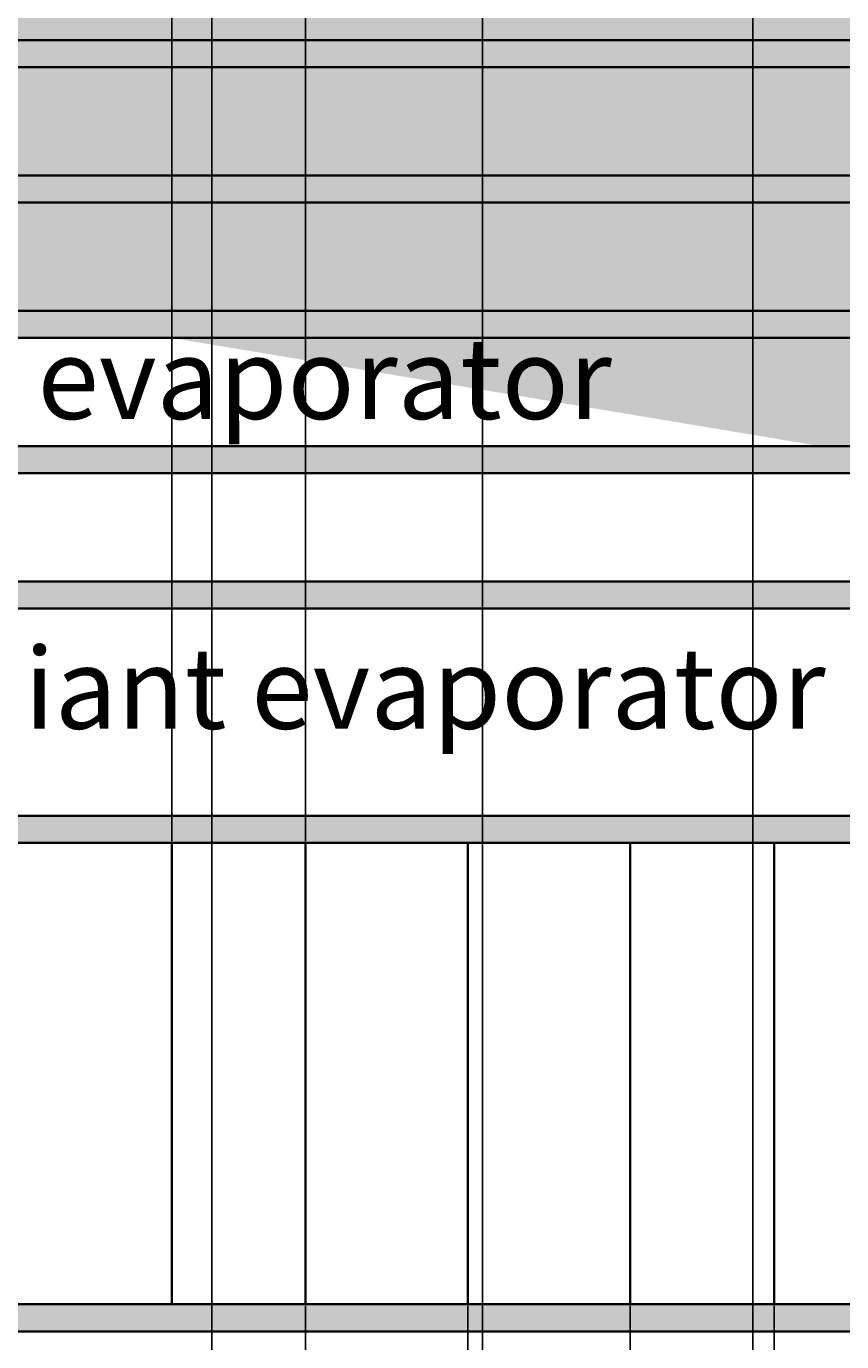
# Model space of a CAD drawing. Units: millimetres. Extents: x -22994 to 29398, y -19990 to 20176.
# Tile 34 of 135: x 139 to 169, y 30 to 78. Entities that reach past the tile are written whole.
import ezdxf

# ---------------------------------------------------------------- set-up
doc = ezdxf.new("R2010")
doc.units = ezdxf.units.MM
doc.header["$MEASUREMENT"] = 0
for name, color, linetype, lineweight in [('M-ANNO-TEXT', 7, 'Continuous', 25), ('M-DIMS', 2, 'Continuous', 18), ('M-EQPM-PATT', 7, 'Continuous', 18), ('M-PIPE', 7, 'Continuous', 35)]:
    doc.layers.add(name, color=color, linetype=linetype, lineweight=lineweight)
doc.styles.get("Standard").update_dxf_attribs({"font": 'arial.ttf'})
doc.dimstyles.get("Standard").update_dxf_attribs({"dimtxt": 0.18, "dimasz": 10000, "dimexe": 0.18, "dimexo": 0.0625, "dimgap": 0.09, "dimtad": 0, "dimtih": 1, "dimtoh": 1, "dimdec": 0, "dimzin": 0, "dimdsep": 46, "dimtxsty": 'Standard', "dimcen": 0.09, "dimadec": 0, "dimazin": 0, "dimtfac": 1, "dimtdec": 0, "dimtofl": 0, "dimtmove": 0, "dimatfit": 3, "dimfxl": 1, "dimtolj": 1, "dimtzin": 0, "dimlwd": 30, "dimarcsym": 0})

# ---------------------------------------------------------------- blocks, each defined once
blk = doc.blocks.new('*D2')
at = {"layer": 'Defpoints', "color": 0, "transparency": 16777216}
for p in [(6.677, 10.271), (290.852, 10.271), (290.852, -5.079)]:
    blk.add_point(p, dxfattribs=at)
at = {"layer": 'M-DIMS', "color": 0, "lineweight": -2, "transparency": 16777216}
for p, q in [((6.677, 10.209), (6.677, -5.259)), ((290.852, 10.209), (290.852, -5.259))]:
    blk.add_line(p, q, dxfattribs=at)
at = {"layer": 'M-DIMS', "color": 0, "lineweight": 30, "transparency": 16777216}
for p, q in [((-9993.323, -5.079), (-19993.323, -5.079)), ((10290.852, -5.079), (20290.852, -5.079))]:
    blk.add_line(p, q, dxfattribs=at)
at = {"layer": 'M-DIMS', "color": 0, "transparency": 16777216}
for points in [[(-9993.323, 1661.588), (-9993.323, -1671.745), (6.677, -5.079)], [(10290.852, 1661.588), (10290.852, -1671.745), (290.852, -5.079)]]:
    blk.add_solid(points, dxfattribs=at)
at = {"layer": 'M-DIMS', "color": 0, "transparency": 16777216, "insert": (148.765, -5.079), "char_height": 0.18, "attachment_point": 5}
blk.add_mtext('\\A1;284.2', dxfattribs=at)
blk = doc.blocks.new('*D3')
at = {"layer": 'Defpoints', "color": 0, "transparency": 16777216}
for p in [(110.265, 204.165), (110.265, 176.366), (95.833, 127.967)]:
    blk.add_point(p, dxfattribs=at)
at = {"layer": 'M-DIMS', "color": 0, "lineweight": 30, "transparency": 16777216}
for p, q in [((-9904.167, 204.165), (-19904.167, 204.165)), ((10110.265, 204.165), (20110.265, 204.165))]:
    blk.add_line(p, q, dxfattribs=at)
at = {"layer": 'M-DIMS', "color": 0, "lineweight": -2, "transparency": 16777216}
for p, q in [((95.833, 128.03), (95.833, 204.345)), ((110.265, 176.429), (110.265, 204.345))]:
    blk.add_line(p, q, dxfattribs=at)
at = {"layer": 'M-DIMS', "color": 0, "transparency": 16777216}
for points in [[(-9904.167, 1870.832), (-9904.167, -1462.501), (95.833, 204.165)], [(10110.265, 1870.832), (10110.265, -1462.501), (110.265, 204.165)]]:
    blk.add_solid(points, dxfattribs=at)
at = {"layer": 'M-DIMS', "color": 0, "transparency": 16777216, "insert": (103.049, 204.165), "char_height": 0.18, "attachment_point": 5}
blk.add_mtext('\\A1;14.432', dxfattribs=at)
blk = doc.blocks.new('*D4')
at = {"layer": 'Defpoints', "color": 0, "transparency": 16777216}
for p in [(116.265, 204.165), (110.265, 176.366), (116.265, 176.366)]:
    blk.add_point(p, dxfattribs=at)
at = {"layer": 'M-DIMS', "color": 0, "lineweight": 30, "transparency": 16777216}
for p, q in [((-9889.735, 204.165), (-19889.735, 204.165)), ((10116.265, 204.165), (20116.265, 204.165))]:
    blk.add_line(p, q, dxfattribs=at)
at = {"layer": 'M-DIMS', "color": 0, "lineweight": -2, "transparency": 16777216}
for p, q in [((110.265, 176.429), (110.265, 204.345)), ((116.265, 176.429), (116.265, 204.345))]:
    blk.add_line(p, q, dxfattribs=at)
at = {"layer": 'M-DIMS', "color": 0, "transparency": 16777216}
for points in [[(-9889.735, 1870.832), (-9889.735, -1462.501), (110.265, 204.165)], [(10116.265, 1870.832), (10116.265, -1462.501), (116.265, 204.165)]]:
    blk.add_solid(points, dxfattribs=at)
at = {"layer": 'M-DIMS', "color": 0, "transparency": 16777216, "insert": (113.265, 204.165), "char_height": 0.18, "attachment_point": 5}
blk.add_mtext('\\A1;6', dxfattribs=at)
blk = doc.blocks.new('*D5')
at = {"layer": 'Defpoints', "color": 0, "transparency": 16777216}
for p in [(181.265, 204.165), (116.265, 176.366), (181.265, 176.366)]:
    blk.add_point(p, dxfattribs=at)
at = {"layer": 'M-DIMS', "color": 0, "lineweight": 30, "transparency": 16777216}
for p, q in [((-9883.735, 204.165), (-19883.735, 204.165)), ((10181.265, 204.165), (20181.265, 204.165))]:
    blk.add_line(p, q, dxfattribs=at)
at = {"layer": 'M-DIMS', "color": 0, "lineweight": -2, "transparency": 16777216}
for p, q in [((116.265, 176.429), (116.265, 204.345)), ((181.265, 176.429), (181.265, 204.345))]:
    blk.add_line(p, q, dxfattribs=at)
at = {"layer": 'M-DIMS', "color": 0, "transparency": 16777216}
for points in [[(-9883.735, 1870.832), (-9883.735, -1462.501), (116.265, 204.165)], [(10181.265, 1870.832), (10181.265, -1462.501), (181.265, 204.165)]]:
    blk.add_solid(points, dxfattribs=at)
at = {"layer": 'M-DIMS', "color": 0, "transparency": 16777216, "insert": (148.765, 204.165), "char_height": 0.18, "attachment_point": 5}
blk.add_mtext('\\A1;65', dxfattribs=at)
blk = doc.blocks.new('*D6')
at = {"layer": 'Defpoints', "color": 0, "transparency": 16777216}
for p in [(187.265, 204.165), (181.265, 176.366), (187.265, 176.366)]:
    blk.add_point(p, dxfattribs=at)
at = {"layer": 'M-DIMS', "color": 0, "lineweight": 30, "transparency": 16777216}
for p, q in [((-9818.735, 204.165), (-19818.735, 204.165)), ((10187.265, 204.165), (20187.265, 204.165))]:
    blk.add_line(p, q, dxfattribs=at)
at = {"layer": 'M-DIMS', "color": 0, "lineweight": -2, "transparency": 16777216}
for p, q in [((181.265, 176.429), (181.265, 204.345)), ((187.265, 176.429), (187.265, 204.345))]:
    blk.add_line(p, q, dxfattribs=at)
at = {"layer": 'M-DIMS', "color": 0, "transparency": 16777216}
for points in [[(-9818.735, 1870.832), (-9818.735, -1462.501), (181.265, 204.165)], [(10187.265, 1870.832), (10187.265, -1462.501), (187.265, 204.165)]]:
    blk.add_solid(points, dxfattribs=at)
at = {"layer": 'M-DIMS', "color": 0, "transparency": 16777216, "insert": (184.265, 204.165), "char_height": 0.18, "attachment_point": 5}
blk.add_mtext('\\A1;6', dxfattribs=at)
blk = doc.blocks.new('*D7')
at = {"layer": 'Defpoints', "color": 0, "transparency": 16777216}
for p in [(201.697, 204.165), (187.265, 176.366), (201.697, 127.967)]:
    blk.add_point(p, dxfattribs=at)
at = {"layer": 'M-DIMS', "color": 0, "lineweight": 30, "transparency": 16777216}
for p, q in [((-9812.735, 204.165), (-19812.735, 204.165)), ((10201.697, 204.165), (20201.697, 204.165))]:
    blk.add_line(p, q, dxfattribs=at)
at = {"layer": 'M-DIMS', "color": 0, "lineweight": -2, "transparency": 16777216}
for p, q in [((187.265, 176.429), (187.265, 204.345)), ((201.697, 128.03), (201.697, 204.345))]:
    blk.add_line(p, q, dxfattribs=at)
at = {"layer": 'M-DIMS', "color": 0, "transparency": 16777216}
for points in [[(-9812.735, 1870.832), (-9812.735, -1462.501), (187.265, 204.165)], [(10201.697, 1870.832), (10201.697, -1462.501), (201.697, 204.165)]]:
    blk.add_solid(points, dxfattribs=at)
at = {"layer": 'M-DIMS', "color": 0, "transparency": 16777216, "insert": (194.481, 204.165), "char_height": 0.18, "attachment_point": 5}
blk.add_mtext('\\A1;14.432', dxfattribs=at)
blk = doc.blocks.new('*D8')
at = {"layer": 'Defpoints', "color": 0, "transparency": 16777216}
for p in [(227.648, 204.165), (227.648, 146.73), (201.697, 127.967)]:
    blk.add_point(p, dxfattribs=at)
at = {"layer": 'M-DIMS', "color": 0, "lineweight": 30, "transparency": 16777216}
for p, q in [((-9798.303, 204.165), (-19798.303, 204.165)), ((10227.648, 204.165), (20227.648, 204.165))]:
    blk.add_line(p, q, dxfattribs=at)
at = {"layer": 'M-DIMS', "color": 0, "lineweight": -2, "transparency": 16777216}
for p, q in [((201.697, 128.03), (201.697, 204.345)), ((227.648, 146.792), (227.648, 204.345))]:
    blk.add_line(p, q, dxfattribs=at)
at = {"layer": 'M-DIMS', "color": 0, "transparency": 16777216}
for points in [[(-9798.303, 1870.832), (-9798.303, -1462.501), (201.697, 204.165)], [(10227.648, 1870.832), (10227.648, -1462.501), (227.648, 204.165)]]:
    blk.add_solid(points, dxfattribs=at)
at = {"layer": 'M-DIMS', "color": 0, "transparency": 16777216, "insert": (214.673, 204.165), "char_height": 0.18, "attachment_point": 5}
blk.add_mtext('\\A1;25.95', dxfattribs=at)
blk = doc.blocks.new('*D9')
at = {"layer": 'Defpoints', "color": 0, "transparency": 16777216}
for p in [(187.265, 176.366), (306.202, 176.366), (290.852, 10.271)]:
    blk.add_point(p, dxfattribs=at)
at = {"layer": 'M-DIMS', "color": 0, "lineweight": 30, "transparency": 16777216}
for p, q in [((306.202, 10176.366), (306.202, 20176.366)), ((306.202, -9989.729), (306.202, -19989.729))]:
    blk.add_line(p, q, dxfattribs=at)
at = {"layer": 'M-DIMS', "color": 0, "lineweight": -2, "transparency": 16777216}
for p, q in [((187.327, 176.366), (306.382, 176.366)), ((290.915, 10.271), (306.382, 10.271))]:
    blk.add_line(p, q, dxfattribs=at)
at = {"layer": 'M-DIMS', "color": 0, "transparency": 16777216}
for points in [[(-1360.465, 10176.366), (1972.869, 10176.366), (306.202, 176.366)], [(-1360.465, -9989.729), (1972.869, -9989.729), (306.202, 10.271)]]:
    blk.add_solid(points, dxfattribs=at)
at = {"layer": 'M-DIMS', "color": 0, "transparency": 16777216, "insert": (306.202, 93.319), "char_height": 0.18, "attachment_point": 5}
blk.add_mtext('\\A1;166.1', dxfattribs=at)
blk = doc.blocks.new('*D10')
at = {"layer": 'Defpoints', "color": 0, "transparency": 16777216}
for p in [(125.65, 136.071), (133.346, 136.071), (133.346, -5.079)]:
    blk.add_point(p, dxfattribs=at)
at = {"layer": 'M-DIMS', "color": 0, "lineweight": -2, "transparency": 16777216}
for p, q in [((125.65, 136.009), (125.65, -5.259)), ((133.346, 136.009), (133.346, -5.259))]:
    blk.add_line(p, q, dxfattribs=at)
at = {"layer": 'M-DIMS', "color": 0, "lineweight": 30, "transparency": 16777216}
for p, q in [((-9874.35, -5.079), (-19874.35, -5.079)), ((10133.346, -5.079), (20133.346, -5.079))]:
    blk.add_line(p, q, dxfattribs=at)
at = {"layer": 'M-DIMS', "color": 0, "transparency": 16777216}
for points in [[(-9874.35, 1661.588), (-9874.35, -1671.745), (125.65, -5.079)], [(10133.346, 1661.588), (10133.346, -1671.745), (133.346, -5.079)]]:
    blk.add_solid(points, dxfattribs=at)
at = {"layer": 'M-DIMS', "color": 0, "transparency": 16777216, "insert": (129.498, -5.079), "char_height": 0.18, "attachment_point": 5}
blk.add_mtext('\\A1;7.696', dxfattribs=at)
blk = doc.blocks.new('*D11')
at = {"layer": 'Defpoints', "color": 0, "transparency": 16777216}
for p in [(133.346, 136.071), (135.65, 136.071), (135.65, -5.079)]:
    blk.add_point(p, dxfattribs=at)
at = {"layer": 'M-DIMS', "color": 0, "lineweight": -2, "transparency": 16777216}
for p, q in [((133.346, 136.009), (133.346, -5.259)), ((135.65, 136.009), (135.65, -5.259))]:
    blk.add_line(p, q, dxfattribs=at)
at = {"layer": 'M-DIMS', "color": 0, "lineweight": 30, "transparency": 16777216}
for p, q in [((-9866.654, -5.079), (-19866.654, -5.079)), ((10135.65, -5.079), (20135.65, -5.079))]:
    blk.add_line(p, q, dxfattribs=at)
at = {"layer": 'M-DIMS', "color": 0, "transparency": 16777216}
for points in [[(-9866.654, 1661.588), (-9866.654, -1671.745), (133.346, -5.079)], [(10135.65, 1661.588), (10135.65, -1671.745), (135.65, -5.079)]]:
    blk.add_solid(points, dxfattribs=at)
at = {"layer": 'M-DIMS', "color": 0, "transparency": 16777216, "insert": (134.498, -5.079), "char_height": 0.18, "attachment_point": 5}
blk.add_mtext('\\A1;2.304', dxfattribs=at)
blk = doc.blocks.new('*D12')
at = {"layer": 'Defpoints', "color": 0, "transparency": 16777216}
for p in [(135.65, 136.071), (145.65, 136.071), (145.65, -5.079)]:
    blk.add_point(p, dxfattribs=at)
at = {"layer": 'M-DIMS', "color": 0, "lineweight": -2, "transparency": 16777216}
for p, q in [((135.65, 136.009), (135.65, -5.259)), ((145.65, 136.009), (145.65, -5.259))]:
    blk.add_line(p, q, dxfattribs=at)
at = {"layer": 'M-DIMS', "color": 0, "lineweight": 30, "transparency": 16777216}
for p, q in [((-9864.35, -5.079), (-19864.35, -5.079)), ((10145.65, -5.079), (20145.65, -5.079))]:
    blk.add_line(p, q, dxfattribs=at)
at = {"layer": 'M-DIMS', "color": 0, "transparency": 16777216}
for points in [[(-9864.35, 1661.588), (-9864.35, -1671.745), (135.65, -5.079)], [(10145.65, 1661.588), (10145.65, -1671.745), (145.65, -5.079)]]:
    blk.add_solid(points, dxfattribs=at)
at = {"layer": 'M-DIMS', "color": 0, "transparency": 16777216, "insert": (140.65, -5.079), "char_height": 0.18, "attachment_point": 5}
blk.add_mtext('\\A1;10', dxfattribs=at)
blk = doc.blocks.new('*D13')
at = {"layer": 'Defpoints', "color": 0, "transparency": 16777216}
for p in [(145.65, 136.071), (155.65, 136.071), (155.65, -5.079)]:
    blk.add_point(p, dxfattribs=at)
at = {"layer": 'M-DIMS', "color": 0, "lineweight": -2, "transparency": 16777216}
for p, q in [((145.65, 136.009), (145.65, -5.259)), ((155.65, 136.009), (155.65, -5.259))]:
    blk.add_line(p, q, dxfattribs=at)
at = {"layer": 'M-DIMS', "color": 0, "lineweight": 30, "transparency": 16777216}
for p, q in [((-9854.35, -5.079), (-19854.35, -5.079)), ((10155.65, -5.079), (20155.65, -5.079))]:
    blk.add_line(p, q, dxfattribs=at)
at = {"layer": 'M-DIMS', "color": 0, "transparency": 16777216}
for points in [[(-9854.35, 1661.588), (-9854.35, -1671.745), (145.65, -5.079)], [(10155.65, 1661.588), (10155.65, -1671.745), (155.65, -5.079)]]:
    blk.add_solid(points, dxfattribs=at)
at = {"layer": 'M-DIMS', "color": 0, "transparency": 16777216, "insert": (150.65, -5.079), "char_height": 0.18, "attachment_point": 5}
blk.add_mtext('\\A1;10', dxfattribs=at)
blk = doc.blocks.new('*D14')
at = {"layer": 'Defpoints', "color": 0, "transparency": 16777216}
for p in [(155.65, 136.071), (165.65, 136.071), (165.65, -5.079)]:
    blk.add_point(p, dxfattribs=at)
at = {"layer": 'M-DIMS', "color": 0, "lineweight": -2, "transparency": 16777216}
for p, q in [((155.65, 136.009), (155.65, -5.259)), ((165.65, 136.009), (165.65, -5.259))]:
    blk.add_line(p, q, dxfattribs=at)
at = {"layer": 'M-DIMS', "color": 0, "lineweight": 30, "transparency": 16777216}
for p, q in [((-9844.35, -5.079), (-19844.35, -5.079)), ((10165.65, -5.079), (20165.65, -5.079))]:
    blk.add_line(p, q, dxfattribs=at)
at = {"layer": 'M-DIMS', "color": 0, "transparency": 16777216}
for points in [[(-9844.35, 1661.588), (-9844.35, -1671.745), (155.65, -5.079)], [(10165.65, 1661.588), (10165.65, -1671.745), (165.65, -5.079)]]:
    blk.add_solid(points, dxfattribs=at)
at = {"layer": 'M-DIMS', "color": 0, "transparency": 16777216, "insert": (160.65, -5.079), "char_height": 0.18, "attachment_point": 5}
blk.add_mtext('\\A1;10', dxfattribs=at)
blk = doc.blocks.new('*D15')
at = {"layer": 'Defpoints', "color": 0, "transparency": 16777216}
for p in [(173.346, 154.788), (173.346, 136.071), (306.202, 136.071)]:
    blk.add_point(p, dxfattribs=at)
at = {"layer": 'M-DIMS', "color": 0, "lineweight": 30, "transparency": 16777216}
for p, q in [((306.202, 10154.788), (306.202, 20154.788)), ((306.202, -9863.929), (306.202, -19863.929))]:
    blk.add_line(p, q, dxfattribs=at)
at = {"layer": 'M-DIMS', "color": 0, "lineweight": -2, "transparency": 16777216}
for p, q in [((173.408, 154.788), (306.382, 154.788)), ((173.408, 136.071), (306.382, 136.071))]:
    blk.add_line(p, q, dxfattribs=at)
at = {"layer": 'M-DIMS', "color": 0, "transparency": 16777216}
for points in [[(-1360.465, 10154.788), (1972.869, 10154.788), (306.202, 154.788)], [(-1360.465, -9863.929), (1972.869, -9863.929), (306.202, 136.071)]]:
    blk.add_solid(points, dxfattribs=at)
at = {"layer": 'M-DIMS', "color": 0, "transparency": 16777216, "insert": (306.202, 145.43), "char_height": 0.18, "attachment_point": 5}
blk.add_mtext('\\A1;18.717', dxfattribs=at)
blk = doc.blocks.new('*D16')
at = {"layer": 'Defpoints', "color": 0, "transparency": 16777216}
for p in [(120.17, 204.165), (110.466, 48.035), (120.17, 48.035)]:
    blk.add_point(p, dxfattribs=at)
at = {"layer": 'M-DIMS', "color": 0, "lineweight": 30, "transparency": 16777216}
for p, q in [((-9889.534, 204.165), (-19889.534, 204.165)), ((10120.17, 204.165), (20120.17, 204.165))]:
    blk.add_line(p, q, dxfattribs=at)
at = {"layer": 'M-DIMS', "color": 0, "lineweight": -2, "transparency": 16777216}
for p, q in [((110.466, 48.097), (110.466, 204.345)), ((120.17, 48.097), (120.17, 204.345))]:
    blk.add_line(p, q, dxfattribs=at)
at = {"layer": 'M-DIMS', "color": 0, "transparency": 16777216}
for points in [[(-9889.534, 1870.832), (-9889.534, -1462.501), (110.466, 204.165)], [(10120.17, 1870.832), (10120.17, -1462.501), (120.17, 204.165)]]:
    blk.add_solid(points, dxfattribs=at)
at = {"layer": 'M-DIMS', "color": 0, "transparency": 16777216, "insert": (115.318, 204.165), "char_height": 0.18, "attachment_point": 5}
blk.add_mtext('\\A1;9.704', dxfattribs=at)
blk = doc.blocks.new('*D17')
at = {"layer": 'Defpoints', "color": 0, "transparency": 16777216}
for p in [(126.17, 204.165), (120.17, 48.035), (126.17, 48.035)]:
    blk.add_point(p, dxfattribs=at)
at = {"layer": 'M-DIMS', "color": 0, "lineweight": 30, "transparency": 16777216}
for p, q in [((-9879.83, 204.165), (-19879.83, 204.165)), ((10126.17, 204.165), (20126.17, 204.165))]:
    blk.add_line(p, q, dxfattribs=at)
at = {"layer": 'M-DIMS', "color": 0, "lineweight": -2, "transparency": 16777216}
for p, q in [((120.17, 48.097), (120.17, 204.345)), ((126.17, 48.097), (126.17, 204.345))]:
    blk.add_line(p, q, dxfattribs=at)
at = {"layer": 'M-DIMS', "color": 0, "transparency": 16777216}
for points in [[(-9879.83, 1870.832), (-9879.83, -1462.501), (120.17, 204.165)], [(10126.17, 1870.832), (10126.17, -1462.501), (126.17, 204.165)]]:
    blk.add_solid(points, dxfattribs=at)
at = {"layer": 'M-DIMS', "color": 0, "transparency": 16777216, "insert": (123.17, 204.165), "char_height": 0.18, "attachment_point": 5}
blk.add_mtext('\\A1;6', dxfattribs=at)
blk = doc.blocks.new('*D18')
at = {"layer": 'Defpoints', "color": 0, "transparency": 16777216}
for p in [(132.17, 204.165), (126.17, 48.035), (132.17, 48.035)]:
    blk.add_point(p, dxfattribs=at)
at = {"layer": 'M-DIMS', "color": 0, "lineweight": 30, "transparency": 16777216}
for p, q in [((-9873.83, 204.165), (-19873.83, 204.165)), ((10132.17, 204.165), (20132.17, 204.165))]:
    blk.add_line(p, q, dxfattribs=at)
at = {"layer": 'M-DIMS', "color": 0, "lineweight": -2, "transparency": 16777216}
for p, q in [((126.17, 48.097), (126.17, 204.345)), ((132.17, 48.097), (132.17, 204.345))]:
    blk.add_line(p, q, dxfattribs=at)
at = {"layer": 'M-DIMS', "color": 0, "transparency": 16777216}
for points in [[(-9873.83, 1870.832), (-9873.83, -1462.501), (126.17, 204.165)], [(10132.17, 1870.832), (10132.17, -1462.501), (132.17, 204.165)]]:
    blk.add_solid(points, dxfattribs=at)
at = {"layer": 'M-DIMS', "color": 0, "transparency": 16777216, "insert": (129.17, 204.165), "char_height": 0.18, "attachment_point": 5}
blk.add_mtext('\\A1;6', dxfattribs=at)
blk = doc.blocks.new('*D19')
at = {"layer": 'Defpoints', "color": 0, "transparency": 16777216}
for p in [(138.17, 204.165), (132.17, 48.035), (138.17, 48.035)]:
    blk.add_point(p, dxfattribs=at)
at = {"layer": 'M-DIMS', "color": 0, "lineweight": 30, "transparency": 16777216}
for p, q in [((-9867.83, 204.165), (-19867.83, 204.165)), ((10138.17, 204.165), (20138.17, 204.165))]:
    blk.add_line(p, q, dxfattribs=at)
at = {"layer": 'M-DIMS', "color": 0, "lineweight": -2, "transparency": 16777216}
for p, q in [((132.17, 48.097), (132.17, 204.345)), ((138.17, 48.097), (138.17, 204.345))]:
    blk.add_line(p, q, dxfattribs=at)
at = {"layer": 'M-DIMS', "color": 0, "transparency": 16777216}
for points in [[(-9867.83, 1870.832), (-9867.83, -1462.501), (132.17, 204.165)], [(10138.17, 1870.832), (10138.17, -1462.501), (138.17, 204.165)]]:
    blk.add_solid(points, dxfattribs=at)
at = {"layer": 'M-DIMS', "color": 0, "transparency": 16777216, "insert": (135.17, 204.165), "char_height": 0.18, "attachment_point": 5}
blk.add_mtext('\\A1;6', dxfattribs=at)
blk = doc.blocks.new('*D20')
at = {"layer": 'Defpoints', "color": 0, "transparency": 16777216}
for p in [(144.17, 204.165), (138.17, 48.035), (144.17, 48.035)]:
    blk.add_point(p, dxfattribs=at)
at = {"layer": 'M-DIMS', "color": 0, "lineweight": 30, "transparency": 16777216}
for p, q in [((-9861.83, 204.165), (-19861.83, 204.165)), ((10144.17, 204.165), (20144.17, 204.165))]:
    blk.add_line(p, q, dxfattribs=at)
at = {"layer": 'M-DIMS', "color": 0, "lineweight": -2, "transparency": 16777216}
for p, q in [((138.17, 48.097), (138.17, 204.345)), ((144.17, 48.097), (144.17, 204.345))]:
    blk.add_line(p, q, dxfattribs=at)
at = {"layer": 'M-DIMS', "color": 0, "transparency": 16777216}
for points in [[(-9861.83, 1870.832), (-9861.83, -1462.501), (138.17, 204.165)], [(10144.17, 1870.832), (10144.17, -1462.501), (144.17, 204.165)]]:
    blk.add_solid(points, dxfattribs=at)
at = {"layer": 'M-DIMS', "color": 0, "transparency": 16777216, "insert": (141.17, 204.165), "char_height": 0.18, "attachment_point": 5}
blk.add_mtext('\\A1;6', dxfattribs=at)
blk = doc.blocks.new('*D21')
at = {"layer": 'Defpoints', "color": 0, "transparency": 16777216}
for p in [(149.116, 204.165), (144.17, 48.035), (149.116, 48.035)]:
    blk.add_point(p, dxfattribs=at)
at = {"layer": 'M-DIMS', "color": 0, "lineweight": 30, "transparency": 16777216}
for p, q in [((-9855.83, 204.165), (-19855.83, 204.165)), ((10149.116, 204.165), (20149.116, 204.165))]:
    blk.add_line(p, q, dxfattribs=at)
at = {"layer": 'M-DIMS', "color": 0, "lineweight": -2, "transparency": 16777216}
for p, q in [((144.17, 48.097), (144.17, 204.345)), ((149.116, 48.097), (149.116, 204.345))]:
    blk.add_line(p, q, dxfattribs=at)
at = {"layer": 'M-DIMS', "color": 0, "transparency": 16777216}
for points in [[(-9855.83, 1870.832), (-9855.83, -1462.501), (144.17, 204.165)], [(10149.116, 1870.832), (10149.116, -1462.501), (149.116, 204.165)]]:
    blk.add_solid(points, dxfattribs=at)
at = {"layer": 'M-DIMS', "color": 0, "transparency": 16777216, "insert": (146.643, 204.165), "char_height": 0.18, "attachment_point": 5}
blk.add_mtext('\\A1;4.945', dxfattribs=at)
blk = doc.blocks.new('*D22')
at = {"layer": 'Defpoints', "color": 0, "transparency": 16777216}
for p in [(149.116, 30.99), (155.116, 30.99), (155.116, -5.079)]:
    blk.add_point(p, dxfattribs=at)
at = {"layer": 'M-DIMS', "color": 0, "lineweight": -2, "transparency": 16777216}
for p, q in [((149.116, 30.927), (149.116, -5.259)), ((155.116, 30.927), (155.116, -5.259))]:
    blk.add_line(p, q, dxfattribs=at)
at = {"layer": 'M-DIMS', "color": 0, "lineweight": 30, "transparency": 16777216}
for p, q in [((-9850.884, -5.079), (-19850.884, -5.079)), ((10155.116, -5.079), (20155.116, -5.079))]:
    blk.add_line(p, q, dxfattribs=at)
at = {"layer": 'M-DIMS', "color": 0, "transparency": 16777216}
for points in [[(-9850.884, 1661.588), (-9850.884, -1671.745), (149.116, -5.079)], [(10155.116, 1661.588), (10155.116, -1671.745), (155.116, -5.079)]]:
    blk.add_solid(points, dxfattribs=at)
at = {"layer": 'M-DIMS', "color": 0, "transparency": 16777216, "insert": (152.116, -5.079), "char_height": 0.18, "attachment_point": 5}
blk.add_mtext('\\A1;6', dxfattribs=at)
blk = doc.blocks.new('*D23')
at = {"layer": 'Defpoints', "color": 0, "transparency": 16777216}
for p in [(155.116, 30.99), (161.116, 30.99), (161.116, -5.079)]:
    blk.add_point(p, dxfattribs=at)
at = {"layer": 'M-DIMS', "color": 0, "lineweight": -2, "transparency": 16777216}
for p, q in [((155.116, 30.927), (155.116, -5.259)), ((161.116, 30.927), (161.116, -5.259))]:
    blk.add_line(p, q, dxfattribs=at)
at = {"layer": 'M-DIMS', "color": 0, "lineweight": 30, "transparency": 16777216}
for p, q in [((-9844.884, -5.079), (-19844.884, -5.079)), ((10161.116, -5.079), (20161.116, -5.079))]:
    blk.add_line(p, q, dxfattribs=at)
at = {"layer": 'M-DIMS', "color": 0, "transparency": 16777216}
for points in [[(-9844.884, 1661.588), (-9844.884, -1671.745), (155.116, -5.079)], [(10161.116, 1661.588), (10161.116, -1671.745), (161.116, -5.079)]]:
    blk.add_solid(points, dxfattribs=at)
at = {"layer": 'M-DIMS', "color": 0, "transparency": 16777216, "insert": (158.116, -5.079), "char_height": 0.18, "attachment_point": 5}
blk.add_mtext('\\A1;6', dxfattribs=at)
blk = doc.blocks.new('*D24')
at = {"layer": 'Defpoints', "color": 0, "transparency": 16777216}
for p in [(161.116, 30.99), (166.439, 30.99), (166.439, -5.079)]:
    blk.add_point(p, dxfattribs=at)
at = {"layer": 'M-DIMS', "color": 0, "lineweight": -2, "transparency": 16777216}
for p, q in [((161.116, 30.927), (161.116, -5.259)), ((166.439, 30.927), (166.439, -5.259))]:
    blk.add_line(p, q, dxfattribs=at)
at = {"layer": 'M-DIMS', "color": 0, "lineweight": 30, "transparency": 16777216}
for p, q in [((-9838.884, -5.079), (-19838.884, -5.079)), ((10166.439, -5.079), (20166.439, -5.079))]:
    blk.add_line(p, q, dxfattribs=at)
at = {"layer": 'M-DIMS', "color": 0, "transparency": 16777216}
for points in [[(-9838.884, 1661.588), (-9838.884, -1671.745), (161.116, -5.079)], [(10166.439, 1661.588), (10166.439, -1671.745), (166.439, -5.079)]]:
    blk.add_solid(points, dxfattribs=at)
at = {"layer": 'M-DIMS', "color": 0, "transparency": 16777216, "insert": (163.777, -5.079), "char_height": 0.18, "attachment_point": 5}
blk.add_mtext('\\A1;5.323', dxfattribs=at)
blk = doc.blocks.new('*D25')
at = {"layer": 'Defpoints', "color": 0, "transparency": 16777216}
for p in [(166.439, 30.99), (172.439, 30.99), (172.439, -5.079)]:
    blk.add_point(p, dxfattribs=at)
at = {"layer": 'M-DIMS', "color": 0, "lineweight": -2, "transparency": 16777216}
for p, q in [((166.439, 30.927), (166.439, -5.259)), ((172.439, 30.927), (172.439, -5.259))]:
    blk.add_line(p, q, dxfattribs=at)
at = {"layer": 'M-DIMS', "color": 0, "lineweight": 30, "transparency": 16777216}
for p, q in [((-9833.561, -5.079), (-19833.561, -5.079)), ((10172.439, -5.079), (20172.439, -5.079))]:
    blk.add_line(p, q, dxfattribs=at)
at = {"layer": 'M-DIMS', "color": 0, "transparency": 16777216}
for points in [[(-9833.561, 1661.588), (-9833.561, -1671.745), (166.439, -5.079)], [(10172.439, 1661.588), (10172.439, -1671.745), (172.439, -5.079)]]:
    blk.add_solid(points, dxfattribs=at)
at = {"layer": 'M-DIMS', "color": 0, "transparency": 16777216, "insert": (169.439, -5.079), "char_height": 0.18, "attachment_point": 5}
blk.add_mtext('\\A1;6', dxfattribs=at)
blk = doc.blocks.new('*D26')
at = {"layer": 'Defpoints', "color": 0, "transparency": 16777216}
for p in [(172.439, 30.99), (178.439, 30.99), (178.439, -5.079)]:
    blk.add_point(p, dxfattribs=at)
at = {"layer": 'M-DIMS', "color": 0, "lineweight": -2, "transparency": 16777216}
for p, q in [((172.439, 30.927), (172.439, -5.259)), ((178.439, 30.927), (178.439, -5.259))]:
    blk.add_line(p, q, dxfattribs=at)
at = {"layer": 'M-DIMS', "color": 0, "lineweight": 30, "transparency": 16777216}
for p, q in [((-9827.561, -5.079), (-19827.561, -5.079)), ((10178.439, -5.079), (20178.439, -5.079))]:
    blk.add_line(p, q, dxfattribs=at)
at = {"layer": 'M-DIMS', "color": 0, "transparency": 16777216}
for points in [[(-9827.561, 1661.588), (-9827.561, -1671.745), (172.439, -5.079)], [(10178.439, 1661.588), (10178.439, -1671.745), (178.439, -5.079)]]:
    blk.add_solid(points, dxfattribs=at)
at = {"layer": 'M-DIMS', "color": 0, "transparency": 16777216, "insert": (175.439, -5.079), "char_height": 0.18, "attachment_point": 5}
blk.add_mtext('\\A1;6', dxfattribs=at)
blk = doc.blocks.new('*D27')
at = {"layer": 'Defpoints', "color": 0, "transparency": 16777216}
for p in [(178.439, 30.99), (188.117, 30.99), (188.117, -5.079)]:
    blk.add_point(p, dxfattribs=at)
at = {"layer": 'M-DIMS', "color": 0, "lineweight": -2, "transparency": 16777216}
for p, q in [((178.439, 30.927), (178.439, -5.259)), ((188.117, 30.927), (188.117, -5.259))]:
    blk.add_line(p, q, dxfattribs=at)
at = {"layer": 'M-DIMS', "color": 0, "lineweight": 30, "transparency": 16777216}
for p, q in [((-9821.561, -5.079), (-19821.561, -5.079)), ((10188.117, -5.079), (20188.117, -5.079))]:
    blk.add_line(p, q, dxfattribs=at)
at = {"layer": 'M-DIMS', "color": 0, "transparency": 16777216}
for points in [[(-9821.561, 1661.588), (-9821.561, -1671.745), (178.439, -5.079)], [(10188.117, 1661.588), (10188.117, -1671.745), (188.117, -5.079)]]:
    blk.add_solid(points, dxfattribs=at)
at = {"layer": 'M-DIMS', "color": 0, "transparency": 16777216, "insert": (183.278, -5.079), "char_height": 0.18, "attachment_point": 5}
blk.add_mtext('\\A1;9.679', dxfattribs=at)
blk = doc.blocks.new('*D28')
at = {"layer": 'Defpoints', "color": 0, "transparency": 16777216}
for p in [(188.117, 48.035), (306.202, 48.035), (188.117, 30.99)]:
    blk.add_point(p, dxfattribs=at)
at = {"layer": 'M-DIMS', "color": 0, "lineweight": 30, "transparency": 16777216}
for p, q in [((306.202, 10048.035), (306.202, 20048.035)), ((306.202, -9969.01), (306.202, -19969.01))]:
    blk.add_line(p, q, dxfattribs=at)
at = {"layer": 'M-DIMS', "color": 0, "lineweight": -2, "transparency": 16777216}
for p, q in [((188.18, 48.035), (306.382, 48.035)), ((188.18, 30.99), (306.382, 30.99))]:
    blk.add_line(p, q, dxfattribs=at)
at = {"layer": 'M-DIMS', "color": 0, "transparency": 16777216}
for points in [[(-1360.465, 10048.035), (1972.869, 10048.035), (306.202, 48.035)], [(-1360.465, -9969.01), (1972.869, -9969.01), (306.202, 30.99)]]:
    blk.add_solid(points, dxfattribs=at)
at = {"layer": 'M-DIMS', "color": 0, "transparency": 16777216, "insert": (306.202, 39.512), "char_height": 0.18, "attachment_point": 5}
blk.add_mtext('\\A1;17.045', dxfattribs=at)
blk = doc.blocks.new('*D29')
at = {"layer": 'Defpoints', "color": 0, "transparency": 16777216}
for p in [(36.801, 80.045), (64.03, 80.045)]:
    blk.add_point(p, dxfattribs=at)
at = {"layer": 'M-DIMS', "color": 0, "lineweight": -2, "transparency": 16777216}
for p, q in [((50.325, 80.045), (50.505, 80.045)), ((50.415, 79.955), (50.415, 80.135))]:
    blk.add_line(p, q, dxfattribs=at)
at = {"layer": 'M-DIMS', "color": 0, "lineweight": 30, "transparency": 16777216}
blk.add_line((20064.03, 80.03), (10064.03, 80.038), dxfattribs=at)
at = {"layer": 'M-DIMS', "color": 0, "transparency": 16777216}
blk.add_solid([(10064.031, 1746.704), (10064.028, -1586.629), (64.03, 80.045)], dxfattribs=at)
at = {"layer": 'M-DIMS', "color": 0, "transparency": 16777216, "insert": (20064.521, 80.03), "char_height": 0.18, "attachment_point": 5}
blk.add_mtext('\\A1;∅27.23', dxfattribs=at)
blk = doc.blocks.new('*D36')
at = {"layer": 'Defpoints', "color": 0, "transparency": 16777216}
for p in [(46.39, 31.303), (46.387, 26.593)]:
    blk.add_point(p, dxfattribs=at)
at = {"layer": 'M-DIMS', "color": 0, "lineweight": 30, "transparency": 16777216}
for p, q in [((57.15, 20031.301), (51.77, 10031.302)), ((10057.15, 20031.301), (57.15, 20031.301))]:
    blk.add_line(p, q, dxfattribs=at)
at = {"layer": 'M-DIMS', "color": 0, "lineweight": -2, "transparency": 16777216}
for p, q in [((46.299, 28.948), (46.479, 28.948)), ((46.389, 28.858), (46.389, 29.038))]:
    blk.add_line(p, q, dxfattribs=at)
at = {"layer": 'M-DIMS', "color": 0, "transparency": 16777216}
blk.add_solid([(-1614.896, 10032.199), (1718.436, 10030.405), (46.39, 31.303)], dxfattribs=at)
at = {"layer": 'M-DIMS', "color": 0, "transparency": 16777216, "insert": (10057.554, 20031.301), "char_height": 0.18, "attachment_point": 5}
blk.add_mtext('\\A1;∅4.71', dxfattribs=at)
blk = doc.blocks.new('*D37')
at = {"layer": 'Defpoints', "color": 0, "transparency": 16777216}
for p in [(54.834, 118.615), (59.494, 118.614)]:
    blk.add_point(p, dxfattribs=at)
at = {"layer": 'M-DIMS', "color": 0, "lineweight": -2, "transparency": 16777216}
for p, q in [((57.074, 118.614), (57.254, 118.614)), ((57.164, 118.524), (57.164, 118.704))]:
    blk.add_line(p, q, dxfattribs=at)
at = {"layer": 'M-DIMS', "color": 0, "lineweight": 30, "transparency": 16777216}
blk.add_line((20059.493, 116.253), (10059.494, 117.434), dxfattribs=at)
at = {"layer": 'M-DIMS', "color": 0, "transparency": 16777216}
blk.add_solid([(10059.69, 1784.1), (10059.297, -1549.233), (59.494, 118.614)], dxfattribs=at)
at = {"layer": 'M-DIMS', "color": 0, "transparency": 16777216, "insert": (20059.985, 116.253), "char_height": 0.18, "attachment_point": 5}
blk.add_mtext('\\A1;∅4.659', dxfattribs=at)

msp = doc.modelspace()

# ---------------------------------------------------------------- hatches: boundary and pattern name
at = {"layer": 'M-EQPM-PATT'}
h = msp.add_hatch(color=256, dxfattribs=at)
h.set_gradient(color1=(19, 155, 72), color2=(88, 186, 72), tint=1, name='CYLINDER')
h.paths.add_polyline_path([(109.4658, 29.9895), (189.1175, 29.9895), (189.1175, 77.6953), (128.1172, 77.6953, 0.4142136), (126.1172, 75.6953), (126.1172, 73.6953, 0.4142136), (128.1172, 71.6953), (178.5136, 71.6953, -0.4142136), (179.5136, 70.6953), (179.5136, 68.6953, -0.4142136), (178.5136, 67.6953), (128.1172, 67.6953, 0.4142136), (126.1172, 65.6953), (126.1172, 63.6953, 0.4142136), (128.1172, 61.6953), (178.5136, 61.6953, -0.4142136), (179.5136, 60.6953), (179.5136, 58.6953, -0.4142136), (178.5136, 57.6953), (109.7466, 57.6953, -0.4142136), (108.7466, 58.6953), (108.7466, 75.5922, 0.4142136), (106.7466, 77.5922), (101.8327, 77.5922), (101.8327, 76.5922), (106.7466, 76.5922, -0.4142136), (107.7466, 75.5922), (107.7466, 58.6953, 0.4142136), (109.7466, 56.6953), (178.5136, 56.6953, 0.4142136), (180.5136, 58.6953), (180.5136, 60.6953, 0.4142136), (178.5136, 62.6953), (128.1172, 62.6953, -0.4142136), (127.1172, 63.6953), (127.1172, 65.6953, -0.4142136), (128.1172, 66.6953), (178.5136, 66.6953, 0.4142136), (180.5136, 68.6953), (180.5136, 70.6953, 0.4142136), (178.5136, 72.6953), (128.1172, 72.6953, -0.4142136), (127.1172, 73.6953), (127.1172, 75.6953, -0.4142136), (128.1172, 76.6953), (188.1175, 76.6953), (188.1175, 49.0349), (110.4658, 49.0349), (110.4658, 51.9576), (101.8327, 51.9576), (101.8327, 50.9576), (109.4658, 50.9576), (109.4658, 48.5349)])
h.paths.add_polyline_path([(110.4658, 48.0349), (188.1175, 48.0349), (188.1175, 30.9895), (110.4658, 30.9895)], flags=16)
h.paths.add_polyline_path([(136.1519, 78.0082), (161.2406, 78.0082), (161.2406, 84.1903), (136.1519, 84.1903)], flags=9)

# ---------------------------------------------------------------- linework, layer by layer
at = {"layer": 'M-PIPE'}
for p, q in [((144.1702, 48.0349), (144.1702, 30.9895)), ((149.1157, 48.0349), (149.1157, 30.9895)), ((155.1157, 48.0349), (155.1157, 30.9895)), ((161.1157, 48.0349), (161.1157, 30.9895)), ((166.4387, 48.0349), (166.4387, 30.9895))]:
    msp.add_line(p, q, dxfattribs=at)
for points in [[(189.1175, 29.9895), (189.1175, 77.6953), (128.1172, 77.6953, 0.4142136), (126.1172, 75.6953), (126.1172, 73.6953, 0.4142136), (128.1172, 71.6953), (178.5136, 71.6953, -0.4142136), (179.5136, 70.6953), (179.5136, 68.6953, -0.4142136), (178.5136, 67.6953), (128.1172, 67.6953, 0.4142136), (126.1172, 65.6953), (126.1172, 63.6953, 0.4142136), (128.1172, 61.6953), (178.5136, 61.6953, -0.4142136), (179.5136, 60.6953), (179.5136, 58.6953, -0.4142136), (178.5136, 57.6953), (109.7466, 57.6953, -0.4142136), (108.7466, 58.6953), (108.7466, 75.5922, 0.4142136), (106.7466, 77.5922), (101.8327, 77.5922)], [(188.1175, 49.0349), (188.1175, 76.6953), (128.1172, 76.6953, 0.4142136), (127.1172, 75.6953), (127.1172, 73.6953, 0.4142136), (128.1172, 72.6953), (178.5136, 72.6953, -0.4142136), (180.5136, 70.6953), (180.5136, 68.6953, -0.4142136), (178.5136, 66.6953), (128.1172, 66.6953, 0.4142136), (127.1172, 65.6953), (127.1172, 63.6953, 0.4142136), (128.1172, 62.6953), (178.5136, 62.6953, -0.4142136), (180.5136, 60.6953), (180.5136, 58.6953, -0.4142136), (178.5136, 56.6953), (109.7466, 56.6953, -0.4142136), (107.7466, 58.6953), (107.7466, 75.5922, 0.4142136), (106.7466, 76.5922), (101.8327, 76.5922)]]:
    msp.add_lwpolyline(points, format="xyb", dxfattribs=at)
for points in [[(189.1175, 29.9895), (109.4658, 29.9895), (109.4658, 49.0349)], [(110.4658, 49.0349), (188.1175, 49.0349)], [(188.1175, 30.9895), (110.4658, 30.9895), (110.4658, 48.0349), (188.1175, 48.0349)]]:
    msp.add_lwpolyline(points, dxfattribs=at)

# ---------------------------------------------------------------- texts
at = {"layer": 'M-ANNO-TEXT', "char_height": 3, "attachment_point": 1}
for s, insert in [('evaporator', (139.2101, 66.6953)), ('radiant evaporator', (132.2925, 55.25))]:
    msp.add_mtext_dynamic_manual_height_columns(s, width=37.883315, gutter_width=1, heights=[0], dxfattribs=dict(at, insert=insert))

# ---------------------------------------------------------------- dimensions: what is measured, and where the dimension line sits
at = {"layer": 'M-DIMS'}
for base, p1, p2, override, picture, middle in [((306.202, 176.3662), (290.852, 10.2713), (187.2647, 176.3662), {"dimdec": 1, "dimlfac": 1, "dimrnd": 0, "dimzin": 0, "dimdsep": 46, "dimlunit": 2}, '*D9', (306.202, 93.3187)), ((306.202, 136.0713), (173.3459, 154.788), (173.3459, 136.0713), {"dimdec": 3, "dimlfac": 1, "dimrnd": 0, "dimzin": 0, "dimdsep": 46, "dimlunit": 2}, '*D15', (306.202, 145.4297)), ((306.202, 48.0349), (188.1175, 30.9895), (188.1175, 48.0349), {"dimdec": 3, "dimlfac": 1, "dimrnd": 0, "dimzin": 0, "dimdsep": 46, "dimlunit": 2}, '*D28', (306.202, 39.5122))]:
    dim = msp.add_linear_dim(base=base, p1=p1, p2=p2, angle=90, dimstyle='Standard', override=override, dxfattribs=at)
    dim.commit()
    dim.dimension.update_dxf_attribs({"geometry": picture, "text_midpoint": middle})
dim = msp.add_diameter_dim_2p(p1=(46.3875, 26.5934), p2=(46.39, 31.3035), dimstyle='Standard', override={"dimdec": 2, "dimlfac": 1, "dimrnd": 0, "dimzin": 0, "dimdsep": 46, "dimlunit": 2}, dxfattribs=at)
dim.commit()
dim.dimension.update_dxf_attribs({"geometry": '*D36', "text_midpoint": (10057.5542, 20031.3006), "dimtype": 163})
for base, p1, p2, override, picture, middle in [((110.2647, 204.1654), (95.8327, 127.967), (110.2647, 176.3662), {"dimdec": 3, "dimlfac": 1, "dimrnd": 0, "dimzin": 0, "dimdsep": 46, "dimlunit": 2}, '*D3', (103.0487, 204.1654)), ((116.2647, 204.1654), (110.2647, 176.3662), (116.2647, 176.3662), {"dimdec": 0, "dimlfac": 1, "dimrnd": 0, "dimzin": 0, "dimdsep": 46, "dimlunit": 2}, '*D4', (113.2647, 204.1654)), ((120.1702, 204.1654), (110.4658, 48.0349), (120.1702, 48.0349), {"dimdec": 3, "dimlfac": 1, "dimrnd": 0, "dimzin": 0, "dimdsep": 46, "dimlunit": 2}, '*D16', (115.318, 204.1654)), ((181.2647, 204.1654), (116.2647, 176.3662), (181.2647, 176.3662), {"dimdec": 0, "dimlfac": 1, "dimrnd": 0, "dimzin": 0, "dimdsep": 46, "dimlunit": 2}, '*D5', (148.7647, 204.1654)), ((126.1702, 204.1654), (120.1702, 48.0349), (126.1702, 48.0349), {"dimdec": 0, "dimlfac": 1, "dimrnd": 0, "dimzin": 0, "dimdsep": 46, "dimlunit": 2}, '*D17', (123.1702, 204.1654)), ((132.1702, 204.1654), (126.1702, 48.0349), (132.1702, 48.0349), {"dimdec": 0, "dimlfac": 1, "dimrnd": 0, "dimzin": 0, "dimdsep": 46, "dimlunit": 2}, '*D18', (129.1702, 204.1654)), ((138.1702, 204.1654), (132.1702, 48.0349), (138.1702, 48.0349), {"dimdec": 0, "dimlfac": 1, "dimrnd": 0, "dimzin": 0, "dimdsep": 46, "dimlunit": 2}, '*D19', (135.1702, 204.1654)), ((144.1702, 204.1654), (138.1702, 48.0349), (144.1702, 48.0349), {"dimdec": 0, "dimlfac": 1, "dimrnd": 0, "dimzin": 0, "dimdsep": 46, "dimlunit": 2}, '*D20', (141.1702, 204.1654)), ((149.11567, 204.16539), (144.17023, 48.03494), (149.11567, 48.03494), {"dimdec": 3, "dimlfac": 1, "dimrnd": 0, "dimzin": 0, "dimdsep": 46, "dimlunit": 2}, '*D21', (146.64295, 204.16539)), ((187.2647, 204.1654), (181.2647, 176.3662), (187.2647, 176.3662), {"dimdec": 0, "dimlfac": 1, "dimrnd": 0, "dimzin": 0, "dimdsep": 46, "dimlunit": 2}, '*D6', (184.2647, 204.1654)), ((201.6967, 204.1654), (187.2647, 176.3662), (201.6967, 127.967), {"dimdec": 3, "dimlfac": 1, "dimrnd": 0, "dimzin": 0, "dimdsep": 46, "dimlunit": 2}, '*D7', (194.4807, 204.1654)), ((227.6485, 204.1654), (201.6967, 127.967), (227.6485, 146.7296), {"dimdec": 2, "dimlfac": 1, "dimrnd": 0, "dimzin": 0, "dimdsep": 46, "dimlunit": 2}, '*D8', (214.6726, 204.1654)), ((290.852, -5.0787), (6.6773, 10.2713), (290.852, 10.2713), {"dimdec": 1, "dimlfac": 1, "dimrnd": 0, "dimzin": 0, "dimdsep": 46, "dimlunit": 2}, '*D2', (148.7647, -5.0787)), ((133.3459, -5.0787), (125.6498, 136.0713), (133.3459, 136.0713), {"dimdec": 3, "dimlfac": 1, "dimrnd": 0, "dimzin": 0, "dimdsep": 46, "dimlunit": 2}, '*D10', (129.4978, -5.0787)), ((135.6498, -5.0787), (133.3459, 136.0713), (135.6498, 136.0713), {"dimdec": 3, "dimlfac": 1, "dimrnd": 0, "dimzin": 0, "dimdsep": 46, "dimlunit": 2}, '*D11', (134.4978, -5.0787)), ((145.6498, -5.0787), (135.6498, 136.0713), (145.6498, 136.0713), {"dimdec": 0, "dimlfac": 1, "dimrnd": 0, "dimzin": 0, "dimdsep": 46, "dimlunit": 2}, '*D12', (140.6498, -5.0787)), ((155.6498, -5.0787), (145.6498, 136.0713), (155.6498, 136.0713), {"dimdec": 0, "dimlfac": 1, "dimrnd": 0, "dimzin": 0, "dimdsep": 46, "dimlunit": 2}, '*D13', (150.6498, -5.0787)), ((155.1157, -5.0787), (149.1157, 30.9895), (155.1157, 30.9895), {"dimdec": 0, "dimlfac": 1, "dimrnd": 0, "dimzin": 0, "dimdsep": 46, "dimlunit": 2}, '*D22', (152.1157, -5.0787)), ((161.1157, -5.0787), (155.1157, 30.9895), (161.1157, 30.9895), {"dimdec": 0, "dimlfac": 1, "dimrnd": 0, "dimzin": 0, "dimdsep": 46, "dimlunit": 2}, '*D23', (158.1157, -5.0787)), ((165.6498, -5.0787), (155.6498, 136.0713), (165.6498, 136.0713), {"dimdec": 0, "dimlfac": 1, "dimrnd": 0, "dimzin": 0, "dimdsep": 46, "dimlunit": 2}, '*D14', (160.6498, -5.0787)), ((166.4387, -5.0787), (161.1157, 30.9895), (166.4387, 30.9895), {"dimdec": 3, "dimlfac": 1, "dimrnd": 0, "dimzin": 0, "dimdsep": 46, "dimlunit": 2}, '*D24', (163.7772, -5.0787)), ((172.4387, -5.0787), (166.4387, 30.9895), (172.4387, 30.9895), {"dimdec": 0, "dimlfac": 1, "dimrnd": 0, "dimzin": 0, "dimdsep": 46, "dimlunit": 2}, '*D25', (169.4387, -5.0787)), ((178.4387, -5.0787), (172.4387, 30.9895), (178.4387, 30.9895), {"dimdec": 0, "dimlfac": 1, "dimrnd": 0, "dimzin": 0, "dimdsep": 46, "dimlunit": 2}, '*D26', (175.4387, -5.0787)), ((188.1175, -5.0787), (178.4387, 30.9895), (188.1175, 30.9895), {"dimdec": 3, "dimlfac": 1, "dimrnd": 0, "dimzin": 0, "dimdsep": 46, "dimlunit": 2}, '*D27', (183.2781, -5.0787))]:
    dim = msp.add_linear_dim(base=base, p1=p1, p2=p2, dimstyle='Standard', override=override, dxfattribs=at)
    dim.commit()
    dim.dimension.update_dxf_attribs({"geometry": picture, "text_midpoint": middle})
for p1, p2, override, picture, middle in [((54.8343, 118.6145), (59.4936, 118.614), {"dimdec": 3, "dimlfac": 1, "dimrnd": 0, "dimzin": 0, "dimdsep": 46, "dimlunit": 2}, '*D37', (20059.4934, 116.2531)), ((36.8006, 80.045), (64.0296, 80.045), {"dimdec": 2, "dimlfac": 1, "dimrnd": 0, "dimzin": 0, "dimdsep": 46, "dimlunit": 2}, '*D29', (20064.0296, 80.0303))]:
    dim = msp.add_diameter_dim_2p(p1=p1, p2=p2, dimstyle='Standard', override=override, dxfattribs=at)
    dim.commit()
    dim.dimension.update_dxf_attribs({"geometry": picture, "text_midpoint": middle})

doc.saveas('drawing.dxf')
